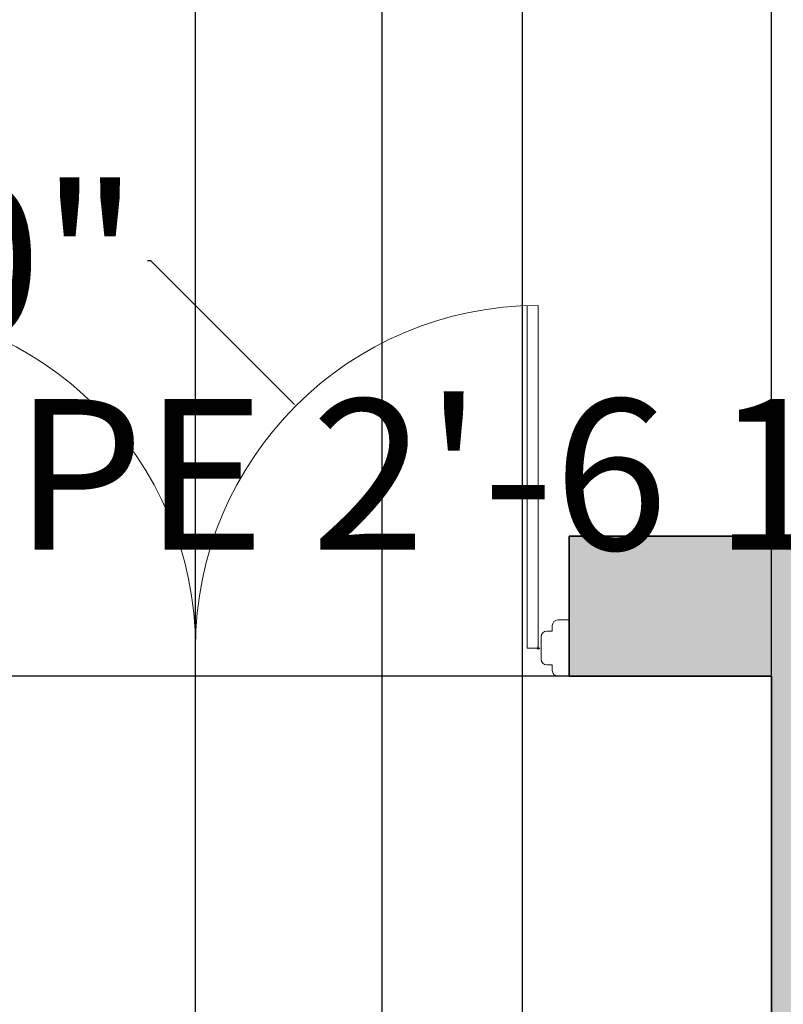
# Model space of a CAD drawing. Units: inches. Extents: x 2103 to 2702, y 2405 to 3142.
# Tile 5 of 7: x 2421 to 2470, y 3039 to 3102. Entities that reach past the tile are written whole.
import ezdxf

# ---------------------------------------------------------------- set-up
doc = ezdxf.new("R2010")
doc.units = ezdxf.units.IN
for name, color, linetype, lineweight in [('00 FURNITURE', 15, 'Continuous', 15), ('A-ANNO-DIMS', 2, 'Continuous', 18), ('A-WALL-PATT', 8, 'Continuous', 9), ('doors', 4, 'Continuous', 18), ('WALL', 7, 'Continuous', 35)]:
    doc.layers.add(name, color=color, linetype=linetype, lineweight=lineweight)
doc.styles.get("Standard").update_dxf_attribs({"font": 'arial.ttf'})
doc.dimstyles.get("Standard").update_dxf_attribs({"dimtxt": 9.68, "dimasz": 0.18, "dimexe": 0.18, "dimexo": 0.0625, "dimgap": 0.09, "dimtad": 0, "dimtih": 1, "dimtoh": 1, "dimdec": 1, "dimzin": 0, "dimdsep": 46, "dimlunit": 3, "dimtxsty": 'Standard', "dimcen": 0.09, "dimadec": 0, "dimazin": 0, "dimtfac": 1, "dimtdec": 1, "dimtofl": 0, "dimtmove": 0, "dimatfit": 3, "dimfxl": 1, "dimtolj": 1, "dimtzin": 0, "dimarcsym": 0})

# ---------------------------------------------------------------- blocks, each defined once
blk = doc.blocks.new('PUJA')
at = {"layer": '00 FURNITURE'}
for p, q in [((-1941.804715046006, -16091.74732686729), (-1938.88804837934, -16091.74732686729)), ((-1941.804715045972, -16092.33066020062), (-1941.804715046006, -16091.74732686729)), ((-1938.88804837934, -16091.74732686729), (-1938.888048379305, -16092.33066020062)), ((-1941.221381712637, -16092.62232686729), (-1941.513048379306, -16092.62232686729)), ((-1939.179715045973, -16092.62232686729), (-1939.471381712639, -16092.62232686729)), ((-1940.346381712639, -16093.35149353396), (-1958.138048379298, -16093.35149353394)), ((-1940.346381712639, -16093.35149353396), (-1940.346381712672, -16093.93482686729)), ((-1940.346381712672, -16093.93482686729), (-1958.128482966474, -16093.93482686727)), ((-1940.346381712672, -16128.35149353396), (-1958.128482966474, -16128.35149353398)), ((-1940.346381712639, -16128.93482686729), (-1940.346381712672, -16128.35149353396)), ((-1940.346381712639, -16128.93482686729), (-1958.138048379298, -16128.93482686731)), ((-1941.221381712637, -16129.66399353396), (-1941.513048379306, -16129.66399353396)), ((-1939.179715045973, -16129.66399353396), (-1939.471381712639, -16129.66399353396)), ((-1941.804715045972, -16129.95566020063), (-1941.804715046006, -16130.53899353396)), ((-1938.88804837934, -16130.53899353396), (-1938.888048379305, -16129.95566020063)), ((-1941.804715046006, -16130.53899353396), (-1938.88804837934, -16130.53899353396))]:
    blk.add_line(p, q, dxfattribs=at)
for points in [[(-1939.471381712639, -16092.62232686729), (-1939.471381712639, -16092.91399353395, -0.4142135623730951), (-1939.763048379305, -16093.20566020062), (-1940.929715045971, -16093.20566020062, -0.4142135623730951), (-1941.221381712637, -16092.91399353395), (-1941.221381712637, -16092.62232686729)], [(-1939.471381712639, -16129.66399353396), (-1939.471381712639, -16129.37232686729, 0.4142135623730951), (-1939.763048379305, -16129.08066020063), (-1940.929715045971, -16129.08066020063, 0.4142135623730951), (-1941.221381712637, -16129.37232686729), (-1941.221381712637, -16129.66399353396)]]:
    blk.add_lwpolyline(points, format="xyb", dxfattribs=at)
for centre, radius, start, end in [((-1941.513048379306, -16092.33066020062), 0.2916666666665321, 180, 270), ((-1939.179715045973, -16092.33066020062), 0.2916666666665321, 270, 0), ((-1940.346381712639, -16093.35149353397), 17.79166666665846, 180, 270), ((-1940.346381712639, -16128.93482686728), 17.79166666665846, 90, 180), ((-1941.513048379306, -16129.95566020063), 0.2916666666665321, 90, 180), ((-1939.179715045973, -16129.95566020063), 0.2916666666665321, 0, 90)]:
    blk.add_arc(centre, radius, start, end, dxfattribs=at)
blk = doc.blocks.new('*D15')
at = {"layer": 'A-ANNO-DIMS', "color": 0, "lineweight": -2, "transparency": 16777216}
for p, q in [((2246.430135310188, 3068.908174366427), (2246.430135310188, 3136.18297836625)), ((2246.610135310187, 3136.002978366251), (2418.129303113734, 3136.002978366251)), ((2606.250135310188, 3136.002978366251), (2434.730967506641, 3136.002978366251)), ((2606.430135310187, 3068.908174366427), (2606.430135310187, 3136.18297836625))]:
    blk.add_line(p, q, dxfattribs=at)
at = {"layer": 'A-ANNO-DIMS', "color": 0, "transparency": 16777216}
for points in [[(2246.610135310187, 3136.032978366251), (2246.610135310187, 3135.97297836625), (2246.430135310188, 3136.002978366251)], [(2606.250135310188, 3136.032978366251), (2606.250135310188, 3135.97297836625), (2606.430135310187, 3136.002978366251)]]:
    blk.add_solid(points, dxfattribs=at)
at = {"layer": 'Defpoints', "color": 0, "transparency": 16777216}
for p in [(2606.430135310187, 3136.002978366251), (2246.430135310188, 3068.845674366427), (2606.430135310187, 3068.845674366427)]:
    blk.add_point(p, dxfattribs=at)
at = {"layer": 'A-ANNO-DIMS', "color": 0, "transparency": 16777216, "insert": (2426.430135310188, 3136.002978366251), "char_height": 9.68, "attachment_point": 5}
blk.add_mtext("\\A1;30'", dxfattribs=at)
blk = doc.blocks.new('*D32')
at = {"layer": 'A-ANNO-DIMS', "color": 0, "lineweight": -2, "transparency": 16777216}
for p, q in [((2523.701954441973, 3069.816092044852), (2527.298623542507, 3072.777740503555)), ((2527.0452500719, 3072.802273835842), (2526.8652500719, 3072.802273835842)), ((2527.15967014106, 3072.663320434396), (2527.0452500719, 3072.802273835842)), ((2546.291633940058, 3049.429184449692), (2527.274090210219, 3072.524367032949)), ((2542.948338310131, 3046.443002658702), (2546.545007410664, 3049.404651117404))]:
    blk.add_line(p, q, dxfattribs=at)
at = {"layer": 'A-ANNO-DIMS', "color": 0, "transparency": 16777216}
for points in [[(2527.297249110461, 3072.543437044476), (2527.250931309978, 3072.505297021422), (2527.15967014106, 3072.663320434396)], [(2546.3147928403, 3049.448254461218), (2546.268475039817, 3049.410114438165), (2546.406054009218, 3049.290231048245)]]:
    blk.add_solid(points, dxfattribs=at)
at = {"layer": 'Defpoints', "color": 0, "transparency": 16777216}
for p in [(2527.15967014106, 3072.663320434396), (2523.653706733137, 3069.776362854172), (2542.900090601295, 3046.403273468022)]:
    blk.add_point(p, dxfattribs=at)
at = {"layer": 'A-ANNO-DIMS', "color": 0, "transparency": 16777216, "insert": (2430.028074082815, 3072.802273835842), "char_height": 9.68, "attachment_point": 5}
blk.add_mtext('\\A1;SINK ENVELOPE 2\'-6 1/2" TYP.', dxfattribs=at)
blk = doc.blocks.new('*D40')
at = {"layer": 'A-ANNO-DIMS', "color": 0, "lineweight": -2, "transparency": 16777216}
for p, q in [((2396.430135, 2906.908174), (2396.430135, 3118.895223)), ((2444.43014, 2842.908175), (2444.43014, 3118.895223)), ((2396.610135, 3118.715223000001), (2407.279400801501, 3118.715223000001)), ((2444.25014, 3118.715223000001), (2433.580874198499, 3118.715223000001))]:
    blk.add_line(p, q, dxfattribs=at)
at = {"layer": 'A-ANNO-DIMS', "color": 0, "transparency": 16777216}
for points in [[(2396.610135, 3118.745223000001), (2396.610135, 3118.685223), (2396.430135, 3118.715223000001)], [(2444.25014, 3118.745223000001), (2444.25014, 3118.685223), (2444.43014, 3118.715223000001)]]:
    blk.add_solid(points, dxfattribs=at)
at = {"layer": 'Defpoints', "color": 0, "transparency": 16777216}
for p in [(2444.43014, 3118.715223000001), (2396.430135, 2906.845674), (2444.43014, 2842.845675)]:
    blk.add_point(p, dxfattribs=at)
at = {"layer": 'A-ANNO-DIMS', "color": 0, "transparency": 16777216, "insert": (2420.4301375, 3118.715223000001), "char_height": 9.68, "attachment_point": 5}
blk.add_mtext('\\A1;4\'-0"', dxfattribs=at)
blk = doc.blocks.new('*D50')
at = {"layer": 'A-ANNO-DIMS', "color": 0, "lineweight": -2, "transparency": 16777216}
for p, q in [((2453.430135, 2569.908174), (2453.430135, 3118.895223)), ((2495.430135, 2569.908174), (2495.430135, 3118.895223)), ((2453.610135, 3118.715223000001), (2461.477488342429, 3118.715223000001)), ((2495.250135, 3118.715223000001), (2487.382781657572, 3118.715223000001))]:
    blk.add_line(p, q, dxfattribs=at)
at = {"layer": 'A-ANNO-DIMS', "color": 0, "transparency": 16777216}
for points in [[(2453.610135, 3118.745223000001), (2453.610135, 3118.685223), (2453.430135, 3118.715223000001)], [(2495.250135, 3118.745223000001), (2495.250135, 3118.685223), (2495.430135, 3118.715223000001)]]:
    blk.add_solid(points, dxfattribs=at)
at = {"layer": 'Defpoints', "color": 0, "transparency": 16777216}
for p in [(2495.430135, 3118.715223000001), (2453.430135, 2569.845674), (2495.430135, 2569.845674)]:
    blk.add_point(p, dxfattribs=at)
at = {"layer": 'A-ANNO-DIMS', "color": 0, "transparency": 16777216, "insert": (2474.430135, 3118.715223000001), "char_height": 9.68, "attachment_point": 5}
blk.add_mtext('\\A1;3\'-6"', dxfattribs=at)
blk = doc.blocks.new('*D64')
at = {"layer": 'A-ANNO-DIMS', "color": 0, "lineweight": -2, "transparency": 16777216}
for p, q in [((2396.430135, 3059.908174), (2396.430135, 3118.895223)), ((2469.430135, 3059.908174), (2469.430135, 3118.895223)), ((2396.610135, 3118.715223000001), (2419.947774836289, 3118.715223000001)), ((2469.250135000001, 3118.715223000001), (2445.912495163711, 3118.715223000001))]:
    blk.add_line(p, q, dxfattribs=at)
at = {"layer": 'A-ANNO-DIMS', "color": 0, "transparency": 16777216}
for points in [[(2396.610135, 3118.745223000001), (2396.610135, 3118.685223), (2396.430135, 3118.715223000001)], [(2469.250135000001, 3118.745223000001), (2469.250135000001, 3118.685223), (2469.430135, 3118.715223000001)]]:
    blk.add_solid(points, dxfattribs=at)
at = {"layer": 'Defpoints', "color": 0, "transparency": 16777216}
for p in [(2469.430135, 3118.715223000001), (2396.430135, 3059.845674), (2469.430135, 3059.845674)]:
    blk.add_point(p, dxfattribs=at)
at = {"layer": 'A-ANNO-DIMS', "color": 0, "transparency": 16777216, "insert": (2432.930135, 3118.715223000001), "char_height": 9.68, "attachment_point": 5}
blk.add_mtext('\\A1;6\'-1"', dxfattribs=at)
blk = doc.blocks.new('*D66')
at = {"layer": 'A-ANNO-DIMS', "color": 0, "lineweight": -2, "transparency": 16777216}
for p, q in [((2384.430135, 2794.908174), (2384.430135, 3118.895223)), ((2432.430135000001, 2794.908174), (2432.430135000001, 3118.895223)), ((2384.610135, 3118.715223000001), (2395.279398301501, 3118.715223000001)), ((2432.250135, 3118.715223000001), (2421.5808716985, 3118.715223000001))]:
    blk.add_line(p, q, dxfattribs=at)
at = {"layer": 'A-ANNO-DIMS', "color": 0, "transparency": 16777216}
for points in [[(2384.610135, 3118.745223000001), (2384.610135, 3118.685223), (2384.430135, 3118.715223000001)], [(2432.250135, 3118.745223000001), (2432.250135, 3118.685223), (2432.430135000001, 3118.715223000001)]]:
    blk.add_solid(points, dxfattribs=at)
at = {"layer": 'Defpoints', "color": 0, "transparency": 16777216}
for p in [(2384.430135, 3118.715223000001), (2384.430135, 2794.845674), (2432.430135000001, 2794.845674)]:
    blk.add_point(p, dxfattribs=at)
at = {"layer": 'A-ANNO-DIMS', "color": 0, "transparency": 16777216, "insert": (2408.430135, 3118.715223000001), "char_height": 9.68, "attachment_point": 5}
blk.add_mtext('\\A1;4\'-0"', dxfattribs=at)
blk = doc.blocks.new('*D68')
at = {"layer": 'A-ANNO-DIMS', "color": 0, "lineweight": -2, "transparency": 16777216}
for p, q in [((2469.367635000001, 3059.845674000001), (2211.200134000002, 3059.845674000001)), ((2211.380134000002, 3059.665674000001), (2211.380134000002, 3034.878020521147)), ((2211.380134000002, 3000.025674000001), (2211.380134000002, 3024.813327478856)), ((2469.367635000001, 2999.845674000001), (2211.200134000002, 2999.845674000001))]:
    blk.add_line(p, q, dxfattribs=at)
at = {"layer": 'A-ANNO-DIMS', "color": 0, "transparency": 16777216}
for points in [[(2211.350134000002, 3059.665674000001), (2211.410134000002, 3059.665674000001), (2211.380134000002, 3059.845674000001)], [(2211.350134000002, 3000.025674000001), (2211.410134000002, 3000.025674000001), (2211.380134000002, 2999.845674000001)]]:
    blk.add_solid(points, dxfattribs=at)
at = {"layer": 'Defpoints', "color": 0, "transparency": 16777216}
for p in [(2469.430135000001, 3059.845674000001), (2211.380134000002, 2999.845674000001), (2469.430135000001, 2999.845674000001)]:
    blk.add_point(p, dxfattribs=at)
at = {"layer": 'A-ANNO-DIMS', "color": 0, "transparency": 16777216, "insert": (2211.380134000002, 3029.845674000001), "char_height": 9.68, "attachment_point": 5}
blk.add_mtext('\\A1;5\'-0"', dxfattribs=at)
blk = doc.blocks.new('*D81')
at = {"layer": 'A-ANNO-DIMS', "color": 0, "lineweight": -2, "transparency": 16777216}
for p, q in [((2429.357713705892, 3086.557070894107), (2429.537713705893, 3086.557070894107)), ((2429.537713705893, 3086.557070894107), (2438.750730311762, 3077.344266752974)), ((2454.355173, 3061.650186), (2454.535173, 3061.650186)), ((2454.445173, 3061.560185999999), (2454.445173, 3061.740186))]:
    blk.add_line(p, q, dxfattribs=at)
at = {"layer": 'A-ANNO-DIMS', "color": 0, "transparency": 16777216}
blk.add_solid([(2438.77194327059, 3077.365480201013), (2438.729517352933, 3077.323053304933), (2438.878011, 3077.216989000001)], dxfattribs=at)
at = {"layer": 'Defpoints', "color": 0, "transparency": 16777216}
for p in [(2438.878011, 3077.216989000001), (2454.445173, 3061.650186)]:
    blk.add_point(p, dxfattribs=at)
at = {"layer": 'A-ANNO-DIMS', "color": 0, "transparency": 16777216, "insert": (2397.414835124719, 3086.557070894106), "char_height": 9.68, "attachment_point": 5}
blk.add_mtext('\\A1;4X R1\'-10"', dxfattribs=at)

msp = doc.modelspace()

# ---------------------------------------------------------------- hatches: boundary and pattern name
at = {"layer": 'A-WALL-PATT'}
h = msp.add_hatch(color=256, dxfattribs=at)
h.dxf.hatch_style = 1
h.paths.add_polyline_path([(2255.430135310187, 3059.845674366427), (2289.470134986133, 3059.845674366427), (2289.470134986133, 3068.845673751283), (2289.470134023053, 3068.845673751283), (2246.430135310188, 3068.845674366427), (2246.430135310188, 3024.226823790437), (2255.430135310187, 3024.226823790437)])
h.paths.add_polyline_path([(2408.430135310188, 3068.845674366427), (2337.470134986133, 3068.845674366427), (2337.470134986133, 3059.845674366427), (2387.430135310188, 3059.845674366427), (2387.430135310188, 3035.845674366427), (2387.430135310188, 2915.845674366427), (2378.430135310188, 2915.845674366427), (2378.430135310188, 2906.845674366427), (2396.430135310188, 2906.845674366428), (2396.430135310188, 3059.845674366427), (2408.430135310191, 3059.845674366426), (2408.43013530998, 3063.454696922708)])
h.paths.add_polyline_path([(2482.430134042344, 3068.845674366426), (2456.430135308767, 3068.845674366427), (2456.430135308769, 3059.845674366427), (2469.430135310187, 3059.845674366427), (2469.430135310187, 2999.845674366426), (2473.430135310187, 2999.845674366426), (2473.430135310187, 3003.845674366429), (2473.430135310187, 3059.845674366427), (2482.430134042344, 3059.845674366427)])
h.paths.add_polyline_path([(2606.430135310187, 3068.845674366427), (2506.430135310187, 3068.845674366426), (2506.430135310186, 3059.845674366427), (2533.430135310188, 3059.845674366427), (2533.430135310188, 3045.845674366427), (2533.774306677458, 3045.845674366427, -0.1430353570515649), (2534.312495590746, 3046.002850129938), (2537.430135310188, 3046.002850129938), (2537.430135310188, 3059.845674366427), (2597.430135310188, 3059.845674366427), (2597.430135310187, 3043.845676685565), (2606.430135310187, 3043.845676685565)])

# ---------------------------------------------------------------- linework, layer by layer
at = {"layer": 'WALL'}
for p, q in [((2456.430135308767, 3068.845674366427), (2482.430135310187, 3068.845674366426)), ((2456.430135308769, 3059.845674369275), (2456.430135308767, 3068.845674366427)), ((2456.430135308772, 3059.845674366427), (2469.430135310187, 3059.845674366427)), ((2469.430135310187, 3059.845674366427), (2469.430135310187, 2999.845674366426))]:
    msp.add_line(p, q, dxfattribs=at)

# ---------------------------------------------------------------- block references
at = {"layer": 'doors', "xscale": 1.237379162154587, "yscale": 1.237379162154587, "zscale": 1.237379162154587, "rotation": 270.0000000034012}
msp.add_blockref('PUJA', (22368.02296037357, 660.7060067360972), dxfattribs=at)

# ---------------------------------------------------------------- dimensions: what is measured, and where the dimension line sits
at = {"layer": 'A-ANNO-DIMS'}
for base, p1, p2, override, picture, middle in [((2606.430135310187, 3136.002978366251), (2246.430135310188, 3068.845674366427), (2606.430135310187, 3068.845674366427), {"dimclrd": 0, "dimclre": 0, "dimclrt": 0}, '*D15', (2426.430135310188, 3136.002978366251)), ((2384.430135, 3118.715223000001), (2432.430135000001, 2794.845674), (2384.430135, 2794.845674), {"dimdec": 1, "dimlfac": 1, "dimrnd": 0, "dimzin": 1, "dimdsep": 46, "dimlunit": 4, "dimfrac": 2}, '*D66', (2408.430135, 3118.715223000001)), ((2444.43014, 3118.715223000001), (2396.430135, 2906.845674), (2444.43014, 2842.845675), {"dimdec": 1, "dimlfac": 1, "dimrnd": 0, "dimzin": 1, "dimdsep": 46, "dimlunit": 4, "dimfrac": 2}, '*D40', (2420.4301375, 3118.715223000001)), ((2469.430135, 3118.715223000001), (2396.430135, 3059.845674), (2469.430135, 3059.845674), {"dimdec": 1, "dimlfac": 1, "dimrnd": 0, "dimzin": 1, "dimdsep": 46, "dimlunit": 4, "dimfrac": 2}, '*D64', (2432.930135, 3118.715223000001)), ((2495.430135, 3118.715223000001), (2453.430135, 2569.845674), (2495.430135, 2569.845674), {"dimdec": 1, "dimlfac": 1, "dimrnd": 0, "dimzin": 1, "dimdsep": 46, "dimlunit": 4, "dimfrac": 2}, '*D50', (2474.430135, 3118.715223000001))]:
    dim = msp.add_linear_dim(base=base, p1=p1, p2=p2, dimstyle='Standard', override=override, dxfattribs=at)
    dim.commit()
    dim.dimension.update_dxf_attribs({"geometry": picture, "text_midpoint": middle})
dim = msp.add_linear_dim(base=(2527.15967014106, 3072.663320434396), p1=(2542.900090601295, 3046.403273468023), p2=(2523.653706733138, 3069.776362854172), angle=129.4694759592849, text='SINK ENVELOPE <> TYP.', dimstyle='Standard', override={"dimdec": 1, "dimlfac": 1, "dimrnd": 0, "dimzin": 1, "dimdsep": 46, "dimlunit": 4, "dimfrac": 2}, dxfattribs=at)
dim.commit()
dim.dimension.update_dxf_attribs({"geometry": '*D32', "text_midpoint": (2430.028074082815, 3072.802273835842)})
dim = msp.add_radius_dim(center=(2454.445173, 3061.650186), mpoint=(2438.878011, 3077.216989000001), text='4X <>', dimstyle='Standard', override={"dimdec": 1, "dimlfac": 1, "dimrnd": 0, "dimzin": 1, "dimdsep": 46, "dimlunit": 4, "dimfrac": 2}, dxfattribs=at)
dim.commit()
dim.dimension.update_dxf_attribs({"geometry": '*D81', "text_midpoint": (2397.414835124719, 3086.557070894106), "dimtype": 164})
dim = msp.add_linear_dim(base=(2211.380134000002, 2999.845674000001), p1=(2469.430135, 3059.845674), p2=(2469.430135, 2999.845674), angle=90, dimstyle='Standard', override={"dimdec": 1, "dimlfac": 1, "dimrnd": 0, "dimzin": 1, "dimdsep": 46, "dimlunit": 4, "dimfrac": 2}, dxfattribs=at)
dim.commit()
dim.dimension.update_dxf_attribs({"geometry": '*D68', "text_midpoint": (2211.380134000002, 3029.845674000001)})

doc.saveas('drawing.dxf')
